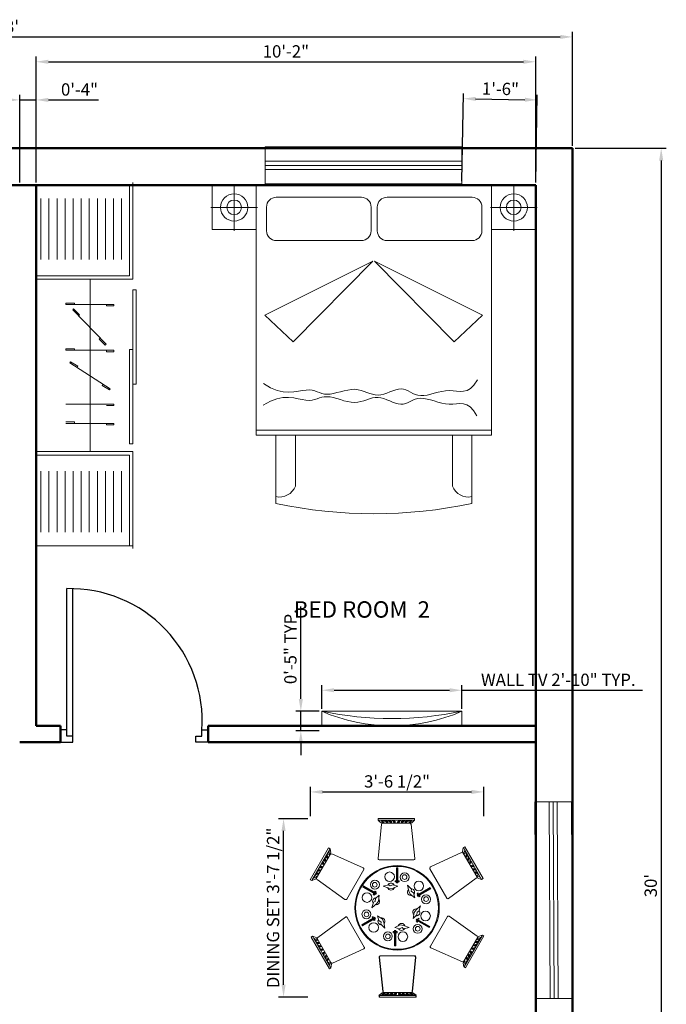
# Model space of a CAD drawing. Units: inches. Extents: x 108 to 1546, y -229 to 513.
# Tile 3 of 11: x 274 to 432, y 147 to 388. Entities that reach past the tile are written whole.
import ezdxf

# ---------------------------------------------------------------- set-up
doc = ezdxf.new("R2010")
doc.units = ezdxf.units.IN
for name, color, linetype, lineweight in [('A-ANNO-DIMS', 2, 'Continuous', 18), ('A-AREA-IDEN', 4, 'Continuous', 18), ('A-FURN', 8, 'Continuous', 13), ('door', 1, 'Continuous', 25), ('tv', 2, 'Continuous', 13), ('wall', 7, 'Continuous', 50), ('WINDOW', 212, 'Continuous', 18)]:
    doc.layers.add(name, color=color, linetype=linetype, lineweight=lineweight)
doc.styles.get("Standard").update_dxf_attribs({"font": 'arial.ttf'})
doc.dimstyles.new('ISO-25', dxfattribs={"dimtxt": 3, "dimasz": 3, "dimexe": 1.25, "dimexo": 0.625, "dimtad": 1, "dimdec": 1, "dimlunit": 3, "dimtxsty": 'Standard', "dimcen": 2.5, "dimadec": 0, "dimazin": 0, "dimtfac": 1, "dimtdec": 1, "dimtmove": 0, "dimatfit": 3, "dimfxl": 1, "dimarcsym": 0})

# ---------------------------------------------------------------- blocks, each defined once
blk = doc.blocks.new('A$C4F543DC7')
for p, q in [((0.013, 3.35, -0.169), (3.313, 3.35, -0.169)), ((0.463, 3.35, -0.169), (0.013, 3.35, -0.169)), ((0.013, 2.896, -0.169), (0.013, 3.35, -0.169)), ((0.013, 3.35, -0.169), (0.013, 2.896, -0.169)), ((0.238, 3.123, -0.439), (0.238, 3.361, -0.439)), ((0.463, 3.35, -0.169), (0.463, 0.8, -0.169)), ((2.863, 3.35, -0.169), (0.463, 3.35, -0.169)), ((0.463, 2.896, -0.169), (0.463, 3.35, -0.169)), ((2.863, 0.8, -0.169), (2.863, 3.35, -0.169)), ((2.863, 3.35, -0.169), (3.313, 3.35, -0.169)), ((2.863, 2.896, -0.169), (2.863, 3.35, -0.169)), ((3.089, 3.123, -0.439), (3.089, 3.361, -0.439)), ((3.313, 3.35, -0.169), (3.313, 2.896, -0.169)), ((3.313, 3.35, -0.169), (3.313, 2.896, -0.169)), ((1.535, 3.226, -0.169), (0.668, 3.226, -0.169)), ((2.664, 3.226, -0.169), (1.797, 3.226, -0.169)), ((0.238, 3.123, -0.439), (0, 3.123, -0.439)), ((0.238, 3.123, -0.439), (0.476, 3.123, -0.439)), ((0.238, 3.123, -0.439), (0.238, 2.885, -0.439)), ((0.568, 3.126, -0.169), (0.568, 2.884, -0.169)), ((1.635, 2.884, -0.169), (1.635, 3.126, -0.169)), ((1.697, 3.126, -0.169), (1.697, 2.884, -0.169)), ((2.764, 2.884, -0.169), (2.764, 3.126, -0.169)), ((3.089, 3.123, -0.439), (2.851, 3.123, -0.439)), ((3.089, 3.123, -0.439), (3.089, 2.885, -0.439)), ((3.089, 3.123, -0.439), (3.327, 3.123, -0.439)), ((0.463, 2.896, -0.169), (0.013, 2.896, -0.169)), ((0.013, 2.896, -0.169), (0.463, 2.896, -0.169)), ((0.463, 0.8, -0.169), (0.463, 2.896, -0.169)), ((2.863, 2.896, -0.169), (2.863, 0.8, -0.169)), ((3.313, 2.896, -0.169), (2.863, 2.896, -0.169)), ((3.313, 2.896, -0.169), (2.863, 2.896, -0.169)), ((0.668, 2.784, -0.169), (1.535, 2.784, -0.169)), ((1.797, 2.784, -0.169), (2.664, 2.784, -0.169)), ((1.653, 2.573, -0.169), (0.55, 2.025, -0.169)), ((0.841, 1.752, -0.169), (1.653, 2.573, -0.169)), ((2.481, 1.752, -0.169), (1.669, 2.573, -0.169)), ((1.669, 2.573, -0.169), (2.772, 2.025, -0.169)), ((0.55, 2.025, -0.169), (0.841, 1.752, -0.169)), ((2.772, 2.025, -0.169), (2.481, 1.752, -0.169)), ((0.537, 1.327, -0.169), (0.609, 1.284, -0.169)), ((2.648, 1.277, -0.169), (2.683, 1.312, -0.169)), ((2.683, 1.312, -0.169), (2.718, 1.364, -0.169)), ((0.609, 1.284, -0.169), (0.676, 1.257, -0.169)), ((0.676, 1.257, -0.169), (0.737, 1.243, -0.169)), ((0.737, 1.243, -0.169), (0.794, 1.239, -0.169)), ((0.794, 1.239, -0.169), (0.846, 1.242, -0.169)), ((0.846, 1.242, -0.169), (0.893, 1.249, -0.169)), ((0.893, 1.249, -0.169), (0.935, 1.256, -0.169)), ((0.935, 1.256, -0.169), (0.972, 1.261, -0.169)), ((0.972, 1.261, -0.169), (1.004, 1.262, -0.169)), ((1.004, 1.262, -0.169), (1.033, 1.258, -0.169)), ((1.033, 1.258, -0.169), (1.06, 1.251, -0.169)), ((1.06, 1.251, -0.169), (1.084, 1.242, -0.169)), ((1.084, 1.242, -0.169), (1.108, 1.234, -0.169)), ((1.108, 1.234, -0.169), (1.132, 1.226, -0.169)), ((1.132, 1.226, -0.169), (1.158, 1.22, -0.169)), ((1.158, 1.22, -0.169), (1.185, 1.218, -0.169)), ((1.185, 1.218, -0.169), (1.216, 1.22, -0.169)), ((1.216, 1.22, -0.169), (1.25, 1.226, -0.169)), ((1.25, 1.226, -0.169), (1.285, 1.235, -0.169)), ((1.285, 1.235, -0.169), (1.322, 1.244, -0.169)), ((1.322, 1.244, -0.169), (1.359, 1.253, -0.169)), ((1.359, 1.253, -0.169), (1.396, 1.261, -0.169)), ((1.396, 1.261, -0.169), (1.433, 1.266, -0.169)), ((1.433, 1.266, -0.169), (1.468, 1.268, -0.169)), ((1.468, 1.268, -0.169), (1.501, 1.264, -0.169)), ((1.501, 1.264, -0.169), (1.532, 1.257, -0.169)), ((1.532, 1.257, -0.169), (1.562, 1.247, -0.169)), ((1.562, 1.247, -0.169), (1.591, 1.237, -0.169)), ((1.591, 1.237, -0.169), (1.62, 1.226, -0.169)), ((1.62, 1.226, -0.169), (1.648, 1.217, -0.169)), ((1.648, 1.217, -0.169), (1.676, 1.211, -0.169)), ((1.676, 1.211, -0.169), (1.705, 1.209, -0.169)), ((1.705, 1.209, -0.169), (1.735, 1.212, -0.169)), ((1.735, 1.212, -0.169), (1.765, 1.22, -0.169)), ((1.765, 1.22, -0.169), (1.795, 1.23, -0.169)), ((1.795, 1.23, -0.169), (1.826, 1.242, -0.169)), ((1.826, 1.242, -0.169), (1.856, 1.253, -0.169)), ((1.856, 1.253, -0.169), (1.885, 1.263, -0.169)), ((1.885, 1.263, -0.169), (1.913, 1.27, -0.169)), ((1.913, 1.27, -0.169), (1.94, 1.272, -0.169)), ((1.94, 1.272, -0.169), (1.965, 1.269, -0.169)), ((1.965, 1.269, -0.169), (1.989, 1.262, -0.169)), ((1.989, 1.262, -0.169), (2.012, 1.251, -0.169)), ((2.012, 1.251, -0.169), (2.036, 1.239, -0.169)), ((2.036, 1.239, -0.169), (2.06, 1.227, -0.169)), ((2.06, 1.227, -0.169), (2.085, 1.216, -0.169)), ((2.085, 1.216, -0.169), (2.112, 1.208, -0.169)), ((2.112, 1.208, -0.169), (2.141, 1.204, -0.169)), ((2.141, 1.204, -0.169), (2.172, 1.205, -0.169)), ((2.172, 1.205, -0.169), (2.206, 1.21, -0.169)), ((2.206, 1.21, -0.169), (2.242, 1.218, -0.169)), ((2.242, 1.218, -0.169), (2.279, 1.228, -0.169)), ((2.279, 1.228, -0.169), (2.317, 1.238, -0.169)), ((2.317, 1.238, -0.169), (2.356, 1.246, -0.169)), ((2.356, 1.246, -0.169), (2.394, 1.253, -0.169)), ((2.394, 1.253, -0.169), (2.433, 1.255, -0.169)), ((2.433, 1.255, -0.169), (2.47, 1.253, -0.169)), ((2.47, 1.253, -0.169), (2.506, 1.249, -0.169)), ((2.506, 1.249, -0.169), (2.542, 1.246, -0.169)), ((2.542, 1.246, -0.169), (2.578, 1.248, -0.169)), ((2.578, 1.248, -0.169), (2.613, 1.257, -0.169)), ((2.613, 1.257, -0.169), (2.648, 1.277, -0.169)), ((0.533, 1.105, -0.169), (0.607, 1.146, -0.169)), ((0.607, 1.146, -0.169), (0.674, 1.171, -0.169)), ((0.674, 1.171, -0.169), (0.736, 1.183, -0.169)), ((0.736, 1.183, -0.169), (0.793, 1.185, -0.169)), ((0.793, 1.185, -0.169), (0.845, 1.18, -0.169)), ((0.845, 1.18, -0.169), (0.891, 1.172, -0.169)), ((0.891, 1.172, -0.169), (0.933, 1.163, -0.169)), ((0.933, 1.163, -0.169), (0.97, 1.156, -0.169)), ((0.97, 1.156, -0.169), (1.003, 1.155, -0.169)), ((1.003, 1.155, -0.169), (1.032, 1.158, -0.169)), ((1.032, 1.158, -0.169), (1.058, 1.164, -0.169)), ((1.058, 1.164, -0.169), (1.083, 1.172, -0.169)), ((1.083, 1.172, -0.169), (1.107, 1.18, -0.169)), ((1.107, 1.18, -0.169), (1.132, 1.187, -0.169)), ((1.132, 1.187, -0.169), (1.157, 1.192, -0.169)), ((1.157, 1.192, -0.169), (1.185, 1.193, -0.169)), ((1.185, 1.193, -0.169), (1.216, 1.19, -0.169)), ((1.216, 1.19, -0.169), (1.249, 1.183, -0.169)), ((1.249, 1.183, -0.169), (1.284, 1.173, -0.169)), ((1.284, 1.173, -0.169), (1.321, 1.163, -0.169)), ((1.321, 1.163, -0.169), (1.358, 1.152, -0.169)), ((1.358, 1.152, -0.169), (1.394, 1.143, -0.169)), ((1.394, 1.143, -0.169), (1.431, 1.137, -0.169)), ((1.431, 1.137, -0.169), (1.466, 1.135, -0.169)), ((1.466, 1.135, -0.169), (1.499, 1.137, -0.169)), ((1.499, 1.137, -0.169), (1.531, 1.143, -0.169)), ((1.531, 1.143, -0.169), (1.561, 1.152, -0.169)), ((1.561, 1.152, -0.169), (1.59, 1.162, -0.169)), ((1.59, 1.162, -0.169), (1.619, 1.172, -0.169)), ((1.619, 1.172, -0.169), (1.648, 1.18, -0.169)), ((1.648, 1.18, -0.169), (1.676, 1.185, -0.169)), ((1.676, 1.185, -0.169), (1.705, 1.186, -0.169)), ((1.705, 1.186, -0.169), (1.734, 1.182, -0.169)), ((1.734, 1.182, -0.169), (1.764, 1.173, -0.169)), ((1.764, 1.173, -0.169), (1.794, 1.162, -0.169)), ((1.794, 1.162, -0.169), (1.824, 1.149, -0.169)), ((1.824, 1.149, -0.169), (1.854, 1.137, -0.169)), ((1.854, 1.137, -0.169), (1.883, 1.126, -0.169)), ((1.883, 1.126, -0.169), (1.911, 1.119, -0.169)), ((1.911, 1.119, -0.169), (1.937, 1.115, -0.169)), ((1.937, 1.115, -0.169), (1.963, 1.118, -0.169)), ((1.963, 1.118, -0.169), (1.987, 1.124, -0.169)), ((1.987, 1.124, -0.169), (2.011, 1.134, -0.169)), ((2.011, 1.134, -0.169), (2.034, 1.145, -0.169)), ((2.034, 1.145, -0.169), (2.059, 1.157, -0.169)), ((2.059, 1.157, -0.169), (2.084, 1.167, -0.169)), ((2.084, 1.167, -0.169), (2.111, 1.174, -0.169)), ((2.111, 1.174, -0.169), (2.14, 1.177, -0.169)), ((2.14, 1.177, -0.169), (2.172, 1.175, -0.169)), ((2.172, 1.175, -0.169), (2.206, 1.169, -0.169)), ((2.206, 1.169, -0.169), (2.241, 1.16, -0.169)), ((2.241, 1.16, -0.169), (2.278, 1.149, -0.169)), ((2.278, 1.149, -0.169), (2.316, 1.138, -0.169)), ((2.316, 1.138, -0.169), (2.354, 1.128, -0.169)), ((2.354, 1.128, -0.169), (2.392, 1.121, -0.169)), ((2.392, 1.121, -0.169), (2.43, 1.117, -0.169)), ((2.43, 1.117, -0.169), (2.468, 1.118, -0.169)), ((2.468, 1.118, -0.169), (2.504, 1.121, -0.169)), ((2.504, 1.121, -0.169), (2.54, 1.123, -0.169)), ((2.54, 1.123, -0.169), (2.576, 1.12, -0.169)), ((2.576, 1.12, -0.169), (2.611, 1.109, -0.169)), ((2.611, 1.109, -0.169), (2.645, 1.088, -0.169)), ((2.645, 1.088, -0.169), (2.679, 1.052, -0.169)), ((2.679, 1.052, -0.169), (2.712, 0.999, -0.169)), ((0.463, 0.85, -0.169), (2.863, 0.85, -0.169)), ((0.463, 0.8, -0.169), (2.863, 0.8, -0.169)), ((0.663, 0.8, -0.169), (0.463, 0.8, -0.169)), ((0.663, 0.8, -0.169), (2.663, 0.8, -0.169)), ((0.663, 0.104, -0.169), (0.663, 0.8, -0.169)), ((0.663, 0.104, -0.169), (0.663, 0.8, -0.169)), ((0.863, 0.281, -0.169), (0.863, 0.8, -0.169)), ((2.463, 0.8, -0.169), (2.463, 0.281, -0.169)), ((2.863, 0.8, -0.169), (2.663, 0.8, -0.169)), ((2.663, 0.8, -0.169), (2.663, 0.104, -0.169)), ((2.663, 0.8, -0.169), (2.663, 0.104, -0.169))]:
    blk.add_line(p, q)
for centre, radius in [((0.238, 3.123, -0.439), 0.139), ((3.089, 3.123, -0.439), 0.139), ((0.238, 3.123, -0.439), 0.075), ((3.089, 3.123, -0.439), 0.075)]:
    blk.add_circle(centre, radius)
for centre, radius, start, end in [((0.668, 3.126, -0.169), 0.1, 90, 180), ((1.535, 3.126, -0.169), 0.1, 0, 90), ((1.797, 3.126, -0.169), 0.1, 90, 180), ((2.664, 3.126, -0.169), 0.1, 0, 90), ((0.668, 2.884, -0.169), 0.1, 180, 270), ((1.535, 2.884, -0.169), 0.1, 270, 0), ((1.797, 2.884, -0.169), 0.1, 180, 270), ((2.664, 2.884, -0.169), 0.1, 270, 0), ((0.699, 0.347, -0.169), 0.177, 258.2616, 338.032), ((2.627, 0.347, -0.169), 0.177, 201.968, 281.7384), ((1.663, 4.86, -0.169), 4.86, 258.1252, 281.8748), ((1.663, 4.86, -0.169), 4.86, 258.1252, 281.8748)]:
    blk.add_arc(centre, radius, start, end)
blk = doc.blocks.new('A$C34930FF8')
for p, q in [((600, 1669.3), (600, 2269.3)), ((580, 1690.9), (580, 2252.4)), ((30, 1790.9), (30, 2169.3)), ((80, 1790.9), (80, 2169.3)), ((130, 1790.9), (130, 2169.3)), ((180, 1790.9), (180, 2169.3)), ((230, 1790.9), (230, 2169.3)), ((280, 1790.9), (280, 2169.3)), ((330, 1790.9), (330, 2169.3)), ((380, 1790.9), (380, 2169.3)), ((430, 1790.9), (430, 2169.3)), ((480, 1790.9), (480, 2169.3)), ((530, 1790.9), (530, 2169.3)), ((580, 1690.9), (0, 1690.9)), ((600, 1669.3), (0, 1669.3)), ((335.4, 1666.1), (335.4, 603.1)), ((600, 1603.3), (620, 1603.3)), ((600, 1018.7), (600, 1603.3)), ((620, 1603.3), (620, 1018.7)), ((237.7, 1521.5), (185.4, 1521.5)), ((482.5, 1513), (185.4, 1513)), ((434.8, 1266.1), (227.4, 1478.9)), ((269.7, 1447.7), (233.2, 1485.2)), ((436.7, 1504.4), (482.5, 1504.4)), ((428.7, 1260.1), (392.1, 1297.6)), ((237.7, 1237.7), (185.4, 1237.7)), ((482.5, 1228.2), (185.4, 1228.2)), ((600, 1233.4), (580, 1233.4)), ((580, 1233.4), (580, 648.7)), ((600, 648.7), (600, 1233.4)), ((436.7, 1219.7), (482.5, 1219.7)), ((459.3, 989.3), (209.5, 1150.1)), ((258.1, 1129), (214.1, 1157.3)), ((454.7, 982.1), (410.6, 1010.5)), ((620, 1018.7), (600, 1018.7)), ((482.5, 894.9), (185.4, 894.9)), ((436.7, 886.3), (482.5, 886.3)), ((237.7, 783.9), (185.4, 783.9)), ((482.5, 775.3), (185.4, 775.3)), ((436.7, 766.8), (482.5, 766.8)), ((580, 648.7), (600, 648.7)), ((600, 600), (0, 600)), ((580, 578.3), (0, 578.3)), ((580, 578.3), (580, 16.8)), ((600, 600), (600, 0)), ((30, 478.3), (30, 100)), ((80, 478.3), (80, 100)), ((130, 478.3), (130, 100)), ((180, 478.3), (180, 100)), ((230, 478.3), (230, 100)), ((280, 478.3), (280, 100)), ((330, 478.3), (330, 100)), ((380, 478.3), (380, 100)), ((430, 478.3), (430, 100)), ((480, 478.3), (480, 100)), ((530, 478.3), (530, 100))]:
    blk.add_line(p, q)
at = {"ltscale": 0.05}
for p, q in [((0, 2252.4), (0, 16.8)), ((600, 2252.4), (0, 2252.4)), ((185.4, 1513), (185.4, 1521.5)), ((227.1, 1479.2), (233.2, 1485.2)), ((237.7, 1513), (237.7, 1521.5)), ((436.7, 1513), (436.7, 1504.4)), ((482.5, 1513), (482.5, 1504.4)), ((263.6, 1441.7), (269.7, 1447.7)), ((398.2, 1303.6), (392.1, 1297.6)), ((185.4, 1229.1), (185.4, 1237.7)), ((237.7, 1229.1), (237.7, 1237.7)), ((434.8, 1266.1), (428.7, 1260.1)), ((436.7, 1228.2), (436.7, 1219.7)), ((482.5, 1228.2), (482.5, 1219.7)), ((209.5, 1150.1), (214.1, 1157.3)), ((253.5, 1121.8), (258.1, 1129)), ((415.3, 1017.6), (410.6, 1010.5)), ((459.3, 989.3), (454.7, 982.1)), ((482.5, 894.9), (482.5, 886.3)), ((237.7, 775.3), (237.7, 783.9)), ((436.7, 775.3), (436.7, 766.8)), ((482.5, 775.3), (482.5, 766.8)), ((600, 16.8), (0, 16.8))]:
    blk.add_line(p, q, dxfattribs=at)
blk = doc.blocks.new('A$C45501D90')
for p, q in [((-242, 1134), (224, 1134)), ((-242, 1113), (-242, 1134)), ((224, 1134), (224, 1113)), ((224, 1113), (-242, 1113)), ((-242, 1111), (-202, 1079)), ((-197, 1062), (-239, 628)), ((-204, 1106), (-166, 1108)), ((-169, 1081), (-204, 1106)), ((-202, 1079), (-169, 1081)), ((162, 1076), (-181, 1076)), ((-166, 1108), (-167, 1086)), ((-156, 1110), (-132, 1086)), ((-119, 1086), (-143, 1108)), ((-143, 1108), (-134, 1108)), ((-134, 1108), (-122, 1098)), ((-132, 1086), (-119, 1086)), ((-122, 1098), (-119, 1102)), ((-119, 1102), (-118, 1087)), ((-108, 1110), (-84, 1086)), ((-71, 1086), (-95, 1108)), ((-95, 1108), (-86, 1108)), ((-86, 1108), (-75, 1098)), ((-84, 1086), (-71, 1086)), ((-75, 1098), (-71, 1102)), ((-71, 1102), (-70, 1087)), ((-60, 1110), (-36, 1086)), ((-23, 1086), (-47, 1108)), ((-47, 1108), (-38, 1108)), ((-38, 1108), (-27, 1098)), ((-36, 1086), (-23, 1086)), ((-27, 1098), (-23, 1102)), ((-23, 1102), (-22, 1087)), ((8, 1102), (7, 1087)), ((8, 1086), (32, 1108)), ((12, 1098), (8, 1102)), ((21, 1086), (8, 1086)), ((23, 1108), (12, 1098)), ((45, 1110), (21, 1086)), ((32, 1108), (23, 1108)), ((56, 1102), (55, 1087)), ((56, 1086), (80, 1108)), ((60, 1098), (56, 1102)), ((69, 1086), (56, 1086)), ((71, 1108), (60, 1098)), ((93, 1110), (69, 1086)), ((80, 1108), (71, 1108)), ((104, 1102), (103, 1087)), ((104, 1086), (128, 1108)), ((107, 1098), (104, 1102)), ((117, 1086), (104, 1086)), ((119, 1108), (107, 1098)), ((141, 1110), (117, 1086)), ((128, 1108), (119, 1108)), ((189, 1106), (151, 1108)), ((151, 1108), (152, 1086)), ((154, 1081), (189, 1106)), ((187, 1079), (154, 1081)), ((225, 628), (178, 1062)), ((224, 1113), (187, 1079)), ((-1103, 357), (-870, 761)), ((-870, 761), (-852, 750)), ((-849, 752), (-841, 702)), ((841, 765), (834, 715)), ((843, 766), (861, 776)), ((1076, 362), (843, 766)), ((861, 776), (1094, 373)), ((-852, 750), (-1085, 347)), ((-851, 678), (-1023, 381)), ((-914, 635), (-906, 603)), ((-898, 642), (-902, 641)), ((-902, 641), (-890, 633)), ((-895, 665), (-900, 657)), ((-900, 657), (-898, 642)), ((-888, 633), (-895, 665)), ((-890, 677), (-882, 644)), ((-882, 644), (-888, 633)), ((-864, 717), (-884, 684)), ((-884, 684), (-864, 675)), ((-859, 674), (-864, 717)), ((-841, 702), (-859, 674)), ((-431, 509), (-831, 685)), ((821, 702), (424, 521)), ((834, 715), (852, 687)), ((1013, 398), (841, 695)), ((852, 687), (856, 730)), ((856, 730), (877, 697)), ((877, 697), (857, 688)), ((883, 690), (874, 657)), ((874, 657), (881, 646)), ((881, 646), (888, 678)), ((894, 654), (883, 646)), ((888, 678), (893, 670)), ((893, 670), (890, 655)), ((890, 655), (894, 654)), ((907, 648), (898, 616)), ((904, 605), (912, 637)), ((912, 637), (917, 628)), ((917, 628), (914, 614)), ((-991, 503), (-958, 511)), ((-952, 522), (-983, 513)), ((-983, 513), (-978, 521)), ((-978, 521), (-965, 526)), ((-965, 526), (-966, 530)), ((-966, 530), (-953, 525)), ((-958, 511), (-952, 522)), ((-945, 559), (-950, 558)), ((-950, 558), (-938, 550)), ((-943, 582), (-948, 574)), ((-948, 574), (-945, 559)), ((-936, 550), (-943, 582)), ((-938, 594), (-930, 561)), ((-930, 561), (-936, 550)), ((-921, 601), (-926, 600)), ((-926, 600), (-914, 591)), ((-919, 624), (-924, 615)), ((-924, 615), (-921, 601)), ((-912, 592), (-919, 624)), ((-906, 603), (-912, 592)), ((-223, 610), (209, 610)), ((-6, 509, 91), (0, 509, 91)), ((-6, 318, 91), (-6, 509, 91)), ((0, 509, 91), (0, 318, 91)), ((6, 318, 91), (6, 509, 91)), ((6, 509, 91), (12, 509, 91)), ((12, 509, 91), (12, 318, 91)), ((898, 616), (904, 605)), ((918, 613), (907, 604)), ((914, 614), (918, 613)), ((931, 607), (922, 574)), ((922, 574), (928, 563)), ((928, 563), (936, 595)), ((942, 571), (931, 563)), ((936, 595), (941, 587)), ((941, 587), (938, 572)), ((938, 572), (942, 571)), ((951, 524), (944, 535)), ((944, 535), (976, 526)), ((958, 543), (945, 538)), ((983, 516), (951, 524)), ((957, 539), (958, 543)), ((971, 534), (957, 539)), ((982, 502), (969, 496)), ((976, 526), (971, 534)), ((981, 498), (982, 502)), ((-1060, 377), (-1042, 411)), ((-1020, 394), (-1060, 377)), ((-1042, 411), (-1024, 398)), ((-1039, 420), (-1006, 428)), ((-1036, 364), (-1020, 394)), ((-1000, 440), (-1031, 430)), ((-1031, 430), (-1026, 438)), ((-1026, 438), (-1012, 443)), ((-1015, 461), (-982, 470)), ((-1012, 443), (-1014, 448)), ((-1014, 448), (-1000, 442)), ((-976, 481), (-1007, 471)), ((-1007, 471), (-1002, 480)), ((-1006, 428), (-1000, 440)), ((-1002, 480), (-989, 485)), ((-989, 485), (-990, 489)), ((-990, 489), (-976, 483)), ((-982, 470), (-976, 481)), ((-640, 112), (-424, 486)), ((417, 498), (633, 124)), ((656, 119), (1008, 377)), ((968, 494), (1000, 484)), ((975, 483), (968, 494)), ((1007, 474), (975, 483)), ((995, 493), (981, 498)), ((999, 441), (992, 453)), ((992, 453), (1024, 443)), ((1006, 461), (993, 455)), ((1000, 484), (995, 493)), ((1031, 433), (999, 441)), ((1005, 456), (1006, 461)), ((1019, 451), (1005, 456)), ((1028, 377), (1013, 407)), ((1013, 407), (1053, 390)), ((1035, 424), (1016, 411)), ((1024, 443), (1019, 451)), ((1076, 359), (1028, 377)), ((1053, 390), (1035, 424)), ((-1085, 347), (-1103, 357)), ((-1083, 346), (-1036, 364)), ((-1018, 360), (-663, 107)), ((-436, 265, 91), (-433, 271, 91)), ((-271, 170, 91), (-436, 265, 91)), ((-433, 271, 91), (-268, 175, 91)), ((-431, 275, 91), (-428, 280, 91)), ((-265, 180, 91), (-431, 275, 91)), ((-428, 280, 91), (-262, 185, 91)), ((-175, 276, 91), (-105, 293, 91)), ((-103, 252, 91), (-175, 276, 91)), ((-105, 293, 91), (-86, 278, 91)), ((-60, 246, 91), (-103, 252, 91)), ((-86, 278, 91), (-52, 294, 91)), ((9, 276, 91), (-60, 246, 91)), ((-52, 294, 91), (9, 276, 91)), ((-22, 329, 91), (-22, 345, 91)), ((-22, 345, 91), (-6, 345, 91)), ((-6, 329, 91), (-22, 329, 91)), ((0, 318, 91), (-6, 318, 91)), ((0, 345, 91), (6, 345, 91)), ((6, 329, 91), (0, 329, 91)), ((12, 318, 91), (6, 318, 91)), ((12, 345, 91), (27, 345, 91)), ((27, 329, 91), (12, 329, 91)), ((27, 345, 91), (27, 329, 91)), ((134, 288, 91), (184, 236, 91)), ((150, 214, 91), (134, 288, 91)), ((255, 162, 91), (421, 257, 91)), ((424, 252, 91), (258, 157, 91)), ((421, 257, 91), (424, 252, 91)), ((1094, 373), (1076, 362)), ((-303, 169, 91), (-294, 183, 91)), ((-289, 161, 91), (-303, 169, 91)), ((-291, 188, 91), (-289, 193, 91)), ((-281, 176, 91), (-289, 161, 91)), ((-286, 198, 91), (-278, 212, 91)), ((-278, 212, 91), (-264, 204, 91)), ((-275, 185, 91), (-278, 181, 91)), ((-274, 118, 91), (-227, 162, 91)), ((-264, 204, 91), (-272, 191, 91)), ((-268, 175, 91), (-271, 170, 91)), ((-262, 185, 91), (-265, 180, 91)), ((-227, 162, 91), (-236, 87, 91)), ((166, 173, 91), (150, 214, 91)), ((227, 128, 91), (166, 173, 91)), ((184, 236, 91), (181, 211, 91)), ((181, 211, 91), (211, 190, 91)), ((211, 190, 91), (227, 128, 91)), ((258, 157, 91), (255, 162, 91)), ((257, 182, 91), (270, 190, 91)), ((265, 168, 91), (257, 182, 91)), ((261, 152, 91), (426, 248, 91)), ((264, 147, 91), (261, 152, 91)), ((429, 242, 91), (264, 147, 91)), ((271, 158, 91), (268, 162, 91)), ((270, 190, 91), (278, 175, 91)), ((281, 139, 91), (274, 153, 91)), ((281, 170, 91), (284, 165, 91)), ((295, 147, 91), (281, 139, 91)), ((287, 160, 91), (295, 147, 91)), ((426, 248, 91), (429, 242, 91)), ((-320, 2, 91), (-299, 72, 91)), ((-263, 53, 91), (-320, 2, 91)), ((-299, 72, 91), (-277, 81, 91)), ((-277, 81, 91), (-274, 118, 91)), ((-236, 87, 91), (-263, 53, 91)), ((243, -25, 91), (299, 26, 91)), ((299, 26, 91), (279, -44, 91)), ((-656, -119), (-1008, -377)), ((-417, -498), (-633, -124)), ((-450, -214, 91), (-284, -119, 91)), ((-281, -124, 91), (-447, -220, 91)), ((-315, -119, 91), (-302, -111, 91)), ((-307, -132, 91), (-315, -119, 91)), ((-302, -111, 91), (-294, -125, 91)), ((-284, -119, 91), (-281, -124, 91)), ((-247, -100, 91), (-187, -145, 91)), ((-232, -162, 91), (-247, -100, 91)), ((207, -134, 91), (216, -60, 91)), ((253, -90, 91), (207, -134, 91)), ((216, -60, 91), (243, -25, 91)), ((256, -53, 91), (253, -90, 91)), ((279, -44, 91), (256, -53, 91)), ((640, -112), (424, -486)), ((1018, -360), (663, -107)), ((-447, -220, 91), (-450, -214, 91)), ((-444, -224, 91), (-279, -129, 91)), ((-441, -229, 91), (-444, -224, 91)), ((-276, -134, 91), (-441, -229, 91)), ((-302, -142, 91), (-304, -137, 91)), ((-290, -162, 91), (-299, -147, 91)), ((-291, -130, 91), (-288, -134, 91)), ((-277, -154, 91), (-290, -162, 91)), ((-285, -140, 91), (-277, -154, 91)), ((-279, -129, 91), (-276, -134, 91)), ((-201, -183, 91), (-232, -162, 91)), ((-205, -208, 91), (-201, -183, 91)), ((-155, -260, 91), (-205, -208, 91)), ((-187, -145, 91), (-170, -186, 91)), ((-170, -186, 91), (-155, -260, 91)), ((-30, -248, 91), (39, -218, 91)), ((32, -266, 91), (-30, -248, 91)), ((65, -250, 91), (32, -266, 91)), ((39, -218, 91), (83, -224, 91)), ((84, -265, 91), (65, -250, 91)), ((83, -224, 91), (155, -248, 91)), ((155, -248, 91), (84, -265, 91)), ((242, -157, 91), (245, -152, 91)), ((407, -252, 91), (242, -157, 91)), ((244, -176, 91), (252, -163, 91)), ((257, -184, 91), (244, -176, 91)), ((245, -152, 91), (410, -247, 91)), ((248, -147, 91), (251, -142, 91)), ((413, -243, 91), (248, -147, 91)), ((251, -142, 91), (416, -237, 91)), ((255, -157, 91), (257, -153, 91)), ((265, -170, 91), (257, -184, 91)), ((260, -148, 91), (269, -133, 91)), ((271, -160, 91), (268, -165, 91)), ((269, -133, 91), (282, -141, 91)), ((282, -141, 91), (274, -155, 91)), ((410, -247, 91), (407, -252, 91)), ((416, -237, 91), (413, -243, 91)), ((-1094, -373), (-1076, -362)), ((-861, -776), (-1094, -373)), ((-1076, -359), (-1028, -377)), ((-1076, -362), (-843, -766)), ((-48, -317, 91), (-48, -301, 91)), ((-48, -301, 91), (-32, -301, 91)), ((-32, -317, 91), (-48, -317, 91)), ((-32, -481, 91), (-32, -290, 91)), ((-32, -290, 91), (-26, -290, 91)), ((-26, -290, 91), (-26, -481, 91)), ((-26, -301, 91), (-21, -301, 91)), ((-21, -317, 91), (-26, -317, 91)), ((-21, -481, 91), (-21, -290, 91)), ((-21, -290, 91), (-15, -290, 91)), ((-15, -290, 91), (-15, -481, 91)), ((-15, -301, 91), (2, -301, 91)), ((2, -317, 91), (-15, -317, 91)), ((2, -301, 91), (2, -317, 91)), ((852, -750), (1085, -347)), ((1103, -357), (870, -761)), ((1036, -364), (1020, -394)), ((1083, -346), (1036, -364)), ((1085, -347), (1103, -357)), ((-1053, -390), (-1035, -424)), ((-1013, -407), (-1053, -390)), ((-1035, -424), (-1016, -411)), ((-1031, -433), (-999, -441)), ((-1028, -377), (-1013, -407)), ((-1024, -443), (-1019, -451)), ((-992, -453), (-1024, -443)), ((-1019, -451), (-1005, -456)), ((-1013, -398), (-841, -695)), ((-1007, -474), (-975, -483)), ((-1006, -461), (-993, -455)), ((-1005, -456), (-1006, -461)), ((-968, -494), (-1000, -484)), ((-1000, -484), (-995, -493)), ((-999, -441), (-992, -453)), ((-995, -493), (-981, -498)), ((-982, -502), (-969, -496)), ((-981, -498), (-982, -502)), ((-975, -483), (-968, -494)), ((-26, -481, 91), (-32, -481, 91)), ((-15, -481, 91), (-21, -481, 91)), ((851, -678), (1023, -381)), ((982, -470), (976, -481)), ((976, -481), (1007, -471)), ((990, -489), (976, -483)), ((1015, -461), (982, -470)), ((1002, -480), (989, -485)), ((989, -485), (990, -489)), ((1006, -428), (1000, -440)), ((1000, -440), (1031, -430)), ((1014, -448), (1000, -442)), ((1007, -471), (1002, -480)), ((1039, -420), (1006, -428)), ((1026, -438), (1012, -443)), ((1012, -443), (1014, -448)), ((1020, -394), (1060, -377)), ((1042, -411), (1024, -398)), ((1031, -430), (1026, -438)), ((1060, -377), (1042, -411)), ((-983, -516), (-951, -524)), ((-944, -535), (-976, -526)), ((-976, -526), (-971, -534)), ((-971, -534), (-957, -539)), ((-958, -543), (-945, -538)), ((-957, -539), (-958, -543)), ((-951, -524), (-944, -535)), ((-942, -571), (-931, -563)), ((-938, -572), (-942, -571)), ((-941, -587), (-938, -572)), ((-936, -595), (-941, -587)), ((-928, -563), (-936, -595)), ((-931, -607), (-922, -574)), ((-922, -574), (-928, -563)), ((-918, -613), (-907, -604)), ((-914, -614), (-918, -613)), ((-917, -628), (-914, -614)), ((-904, -605), (-912, -637)), ((-907, -648), (-898, -616)), ((-898, -616), (-904, -605)), ((-821, -702), (-424, -521)), ((219, -612), (-213, -612)), ((223, -610), (-209, -610)), ((431, -509), (831, -685)), ((906, -603), (912, -592)), ((914, -635), (906, -603)), ((912, -592), (919, -624)), ((926, -600), (914, -591)), ((919, -624), (924, -615)), ((921, -601), (926, -600)), ((924, -615), (921, -601)), ((930, -561), (936, -550)), ((938, -594), (930, -561)), ((936, -550), (943, -582)), ((950, -558), (938, -550)), ((943, -582), (948, -574)), ((945, -559), (950, -558)), ((948, -574), (945, -559)), ((958, -511), (952, -522)), ((952, -522), (983, -513)), ((966, -530), (953, -525)), ((991, -503), (958, -511)), ((978, -521), (965, -526)), ((965, -526), (966, -530)), ((983, -513), (978, -521)), ((-912, -637), (-917, -628)), ((-894, -654), (-883, -646)), ((-890, -655), (-894, -654)), ((-893, -670), (-890, -655)), ((-888, -678), (-893, -670)), ((-881, -646), (-888, -678)), ((-883, -690), (-874, -657)), ((-874, -657), (-881, -646)), ((-877, -697), (-857, -688)), ((-856, -730), (-877, -697)), ((-852, -687), (-856, -730)), ((-834, -715), (-852, -687)), ((-841, -765), (-834, -715)), ((-229, -629), (-182, -1063)), ((-225, -628), (-178, -1062)), ((193, -1063), (235, -629)), ((197, -1062), (239, -628)), ((841, -702), (859, -674)), ((849, -752), (841, -702)), ((870, -761), (852, -750)), ((859, -674), (864, -717)), ((884, -684), (864, -675)), ((864, -717), (884, -684)), ((882, -644), (888, -633)), ((890, -677), (882, -644)), ((888, -633), (895, -665)), ((902, -641), (890, -633)), ((895, -665), (900, -657)), ((898, -642), (902, -641)), ((900, -657), (898, -642)), ((-843, -766), (-861, -776)), ((-231, -1113), (-191, -1081)), ((-228, -1114), (238, -1114)), ((-228, -1135), (-228, -1114)), ((-227, -1111), (-187, -1079)), ((-224, -1113), (242, -1113)), ((-224, -1134), (-224, -1113)), ((-158, -1082), (-193, -1108)), ((-193, -1108), (-155, -1109)), ((-191, -1081), (-158, -1082)), ((-154, -1081), (-189, -1106)), ((-189, -1106), (-151, -1108)), ((-187, -1079), (-154, -1081)), ((-166, -1078), (177, -1078)), ((-162, -1076), (181, -1076)), ((-155, -1109), (-156, -1087)), ((-151, -1108), (-152, -1086)), ((-145, -1111), (-121, -1087)), ((-141, -1110), (-117, -1086)), ((-108, -1087), (-132, -1109)), ((-132, -1109), (-123, -1109)), ((-104, -1086), (-128, -1108)), ((-128, -1108), (-119, -1108)), ((-123, -1109), (-112, -1100)), ((-121, -1087), (-108, -1087)), ((-119, -1108), (-107, -1098)), ((-117, -1086), (-104, -1086)), ((-112, -1100), (-108, -1103)), ((-108, -1103), (-107, -1089)), ((-107, -1098), (-104, -1102)), ((-104, -1102), (-103, -1087)), ((-97, -1111), (-73, -1087)), ((-93, -1110), (-69, -1086)), ((-60, -1087), (-84, -1109)), ((-84, -1109), (-75, -1109)), ((-56, -1086), (-80, -1108)), ((-80, -1108), (-71, -1108)), ((-75, -1109), (-64, -1100)), ((-73, -1087), (-60, -1087)), ((-71, -1108), (-60, -1098)), ((-69, -1086), (-56, -1086)), ((-64, -1100), (-60, -1103)), ((-60, -1103), (-59, -1089)), ((-60, -1098), (-56, -1102)), ((-56, -1102), (-55, -1087)), ((-49, -1111), (-25, -1087)), ((-45, -1110), (-21, -1086)), ((-13, -1087), (-37, -1109)), ((-37, -1109), (-27, -1109)), ((-8, -1086), (-32, -1108)), ((-32, -1108), (-23, -1108)), ((-27, -1109), (-16, -1100)), ((-25, -1087), (-13, -1087)), ((-23, -1108), (-12, -1098)), ((-21, -1086), (-8, -1086)), ((-16, -1100), (-13, -1103)), ((-13, -1103), (-11, -1089)), ((-12, -1098), (-8, -1102)), ((-8, -1102), (-7, -1087)), ((19, -1103), (18, -1089)), ((19, -1087), (43, -1109)), ((32, -1087), (19, -1087)), ((23, -1100), (19, -1103)), ((23, -1102), (22, -1087)), ((23, -1086), (47, -1108)), ((36, -1086), (23, -1086)), ((27, -1098), (23, -1102)), ((34, -1109), (23, -1100)), ((38, -1108), (27, -1098)), ((56, -1111), (32, -1087)), ((43, -1109), (34, -1109)), ((60, -1110), (36, -1086)), ((47, -1108), (38, -1108)), ((67, -1103), (66, -1089)), ((67, -1087), (91, -1109)), ((80, -1087), (67, -1087)), ((70, -1100), (67, -1103)), ((71, -1102), (70, -1087)), ((82, -1109), (70, -1100)), ((71, -1086), (95, -1108)), ((84, -1086), (71, -1086)), ((75, -1098), (71, -1102)), ((86, -1108), (75, -1098)), ((104, -1111), (80, -1087)), ((91, -1109), (82, -1109)), ((108, -1110), (84, -1086)), ((95, -1108), (86, -1108)), ((115, -1103), (114, -1089)), ((115, -1087), (139, -1109)), ((128, -1087), (115, -1087)), ((118, -1100), (115, -1103)), ((119, -1102), (118, -1087)), ((130, -1109), (118, -1100)), ((119, -1086), (143, -1108)), ((132, -1086), (119, -1086)), ((122, -1098), (119, -1102)), ((134, -1108), (122, -1098)), ((152, -1111), (128, -1087)), ((139, -1109), (130, -1109)), ((156, -1110), (132, -1086)), ((143, -1108), (134, -1108)), ((161, -1109), (163, -1087)), ((200, -1108), (161, -1109)), ((198, -1081), (165, -1082)), ((165, -1082), (200, -1108)), ((166, -1108), (167, -1086)), ((204, -1106), (166, -1108)), ((202, -1079), (169, -1081)), ((169, -1081), (204, -1106)), ((238, -1113), (198, -1081)), ((242, -1111), (202, -1079)), ((238, -1114), (238, -1135)), ((242, -1113), (242, -1134)), ((238, -1135), (-228, -1135)), ((242, -1134), (-224, -1134))]:
    blk.add_line(p, q)
for centre, radius in [((0, 0), 537), ((0, 0), 527), ((-95, 395, 91), 61.3), ((97, 390, 91), 56.9), ((96, 391, 91), 29.4), ((-282, 295, 91), 56.9), ((-284, 294, 91), 29.4), ((277, 278, 91), 61.3), ((-382, 131, 91), 61.3), ((369, 109, 91), 56.9), ((369, 111, 91), 29.4), ((-389, -81, 91), 56.9), ((-389, -83, 91), 29.4), ((362, -103, 91), 61.3), ((-298, -250, 91), 61.3), ((262, -267, 91), 56.9), ((263, -266, 91), 29.4), ((-117, -362, 91), 56.9), ((-116, -363, 91), 29.4), ((74, -367, 91), 61.3)]:
    blk.add_circle(centre, radius)
for centre, radius, start, end in [((-181, 1060), 16, 90, 174.5199), ((162, 1060), 16, 6.2572, 90), ((-837, 670), 16, 66.2572, 150), ((-223, 626), 16, 174.5199, 270), ((209, 626), 16, 270, 6.2572), ((827, 687), 16, 30, 114.5199), ((-438, 494), 16, 330, 66.2572), ((431, 506), 16, 114.5199, 210), ((-1009, 373), 16, 150, 234.5199), ((999, 390), 16, 306.2572, 30), ((-77, 270, 91), 44.6, 195.9338, 342.9389), ((-77, 270, 91), 44.6, 25.8558, 153.3359), ((-266, 84, 91), 44.6, 85.8558, 213.3359), ((178, 200, 91), 44.6, 135.9338, 282.9389), ((178, 200, 91), 44.6, 325.8558, 93.3359), ((-654, 120), 16, 234.5199, 330), ((-266, 84, 91), 44.6, 255.9338, 42.9389), ((647, 132), 16, 210, 306.2572), ((-647, -132), 16, 30, 126.2572), ((245, -56, 91), 44.6, 75.9338, 222.9389), ((245, -56, 91), 44.6, 265.8558, 33.3359), ((654, -120), 16, 54.5199, 150), ((-198, -172, 91), 44.6, 145.8558, 273.3359), ((-198, -172, 91), 44.6, 315.9338, 102.9389), ((57, -242, 91), 44.6, 15.9338, 162.9389), ((57, -242, 91), 44.6, 205.8558, 333.3359), ((1009, -373), 16, 330, 54.5199), ((-999, -390), 16, 126.2572, 210), ((-431, -506), 16, 294.5199, 30), ((438, -494), 16, 150, 246.2572), ((-213, -628), 16, 90, 186.2572), ((-209, -626), 16, 90, 186.2572), ((219, -628), 16, 354.5199, 90), ((223, -626), 16, 354.5199, 90), ((-827, -687), 16, 210, 294.5199), ((837, -670), 16, 246.2572, 330), ((-166, -1062), 16, 186.2572, 270), ((-162, -1060), 16, 186.2572, 270), ((177, -1062), 16, 270, 354.5199), ((181, -1060), 16, 270, 354.5199)]:
    blk.add_arc(centre, radius, start, end)
blk = doc.blocks.new('*D21')
at = {"layer": 'A-ANNO-DIMS', "color": 0, "lineweight": -2, "transparency": 16777216}
for p, q in [((132.92, 357.09), (132.92, 384.9)), ((408.92, 357.09), (408.92, 384.9)), ((135.92, 383.65), (405.92, 383.65))]:
    blk.add_line(p, q, dxfattribs=at)
at = {"layer": 'A-ANNO-DIMS', "color": 0, "transparency": 16777216}
for points in [[(135.92, 384.15), (135.92, 383.15), (132.92, 383.65)], [(405.92, 384.15), (405.92, 383.15), (408.92, 383.65)]]:
    blk.add_solid(points, dxfattribs=at)
at = {"layer": 'Defpoints', "color": 0, "transparency": 16777216}
for p in [(408.92, 383.65), (132.92, 356.47), (408.92, 356.47)]:
    blk.add_point(p, dxfattribs=at)
at = {"layer": 'A-ANNO-DIMS', "color": 0, "transparency": 16777216, "insert": (270.92, 385.81), "char_height": 3, "attachment_point": 5}
blk.add_mtext("23'", dxfattribs=at)
blk = doc.blocks.new('*D22')
at = {"layer": 'A-ANNO-DIMS', "color": 0, "lineweight": -2, "transparency": 16777216}
for p, q in [((409.55, 356.47), (431.8, 356.47)), ((430.55, 353.47), (430.55, -0.53)), ((409.55, -3.53), (431.8, -3.53))]:
    blk.add_line(p, q, dxfattribs=at)
at = {"layer": 'A-ANNO-DIMS', "color": 0, "transparency": 16777216}
for points in [[(430.05, 353.47), (431.05, 353.47), (430.55, 356.47)], [(430.05, -0.53), (431.05, -0.53), (430.55, -3.53)]]:
    blk.add_solid(points, dxfattribs=at)
at = {"layer": 'Defpoints', "color": 0, "transparency": 16777216}
for p in [(408.92, 356.47), (408.92, -3.53), (430.55, -3.53)]:
    blk.add_point(p, dxfattribs=at)
at = {"layer": 'A-ANNO-DIMS', "color": 0, "transparency": 16777216, "insert": (428.39, 176.47), "char_height": 3, "attachment_point": 5, "rotation": 90}
blk.add_mtext("30'", dxfattribs=at)
blk = doc.blocks.new('WINDOW-48X9')
for p, q in [((0, 9), (0, 0)), ((0, 9), (48, 9)), ((48, 9), (48, 0)), ((0, 5.5), (48, 5.5)), ((0, 4.5), (48, 4.5)), ((0, 3.5), (48, 3.5)), ((0, 0), (48, 0))]:
    blk.add_line(p, q)
blk = doc.blocks.new('DOOR-SWING-36')
for p, q in [((1.5, 1.5), (1.5, 37.5)), ((3, 1.5), (3, 37.5)), ((0, 3), (0, 0)), ((1.5, 3), (0, 3)), ((1.5, 1.5), (1.5, 3)), ((34.5, 1.5), (34.5, 3)), ((34.5, 3), (36, 3)), ((36, 3), (36, 0)), ((3, 1.5), (1.5, 1.5)), ((3, 0), (3, 1.5)), ((33, 0), (33, 1.5)), ((33, 1.5), (34.5, 1.5)), ((0, 0), (3, 0)), ((36, 0), (33, 0))]:
    blk.add_line(p, q)
blk.add_arc((2.25, 5.18), 32.32, 356.1244, 91.3295)
blk = doc.blocks.new('TV-WALL-MOUNT')
blk.add_lwpolyline([(0, 0), (34.19, 0), (34.19, 3.56), (0, 3.56)], close=True)
for centre, radius, start, end in [((17.1, 42.8), 42.8, 246.4582, 293.5418), ((17.1, 84.72), 82.93, 258.1036, 281.8964)]:
    blk.add_arc(centre, radius, start, end)
blk = doc.blocks.new('*D42')
at = {"layer": 'A-ANNO-DIMS', "color": 0, "lineweight": -2, "transparency": 16777216}
for p, q in [((347.7, 219.66), (347.7, 225.41)), ((350.7, 224.16), (378.89, 224.16)), ((381.89, 219.66), (381.89, 225.41)), ((381.89, 224.16), (425.98, 224.16))]:
    blk.add_line(p, q, dxfattribs=at)
at = {"layer": 'A-ANNO-DIMS', "color": 0, "transparency": 16777216}
for points in [[(350.7, 224.66), (350.7, 223.66), (347.7, 224.16)], [(378.89, 224.66), (378.89, 223.66), (381.89, 224.16)]]:
    blk.add_solid(points, dxfattribs=at)
at = {"layer": 'Defpoints', "color": 0, "transparency": 16777216}
for p in [(381.89, 224.16), (347.7, 219.03), (381.89, 219.03)]:
    blk.add_point(p, dxfattribs=at)
at = {"layer": 'A-ANNO-DIMS', "color": 0, "transparency": 16777216, "insert": (405.43, 226.32), "char_height": 3, "attachment_point": 5}
blk.add_mtext('WALL TV 2\'-10" TYP.', dxfattribs=at)
blk = doc.blocks.new('*D43')
at = {"layer": 'A-ANNO-DIMS', "color": 0, "lineweight": -2, "transparency": 16777216}
for p, q in [((342.57, 222.03), (342.57, 244.57)), ((347.07, 219.03), (341.32, 219.03)), ((342.57, 214.28), (342.57, 219.03)), ((347.07, 214.28), (341.32, 214.28)), ((342.57, 211.28), (342.57, 208.28))]:
    blk.add_line(p, q, dxfattribs=at)
at = {"layer": 'A-ANNO-DIMS', "color": 0, "transparency": 16777216}
for points in [[(342.07, 222.03), (343.07, 222.03), (342.57, 219.03)], [(342.07, 211.28), (343.07, 211.28), (342.57, 214.28)]]:
    blk.add_solid(points, dxfattribs=at)
at = {"layer": 'Defpoints', "color": 0, "transparency": 16777216}
for p in [(342.57, 219.03), (347.7, 219.03), (347.7, 214.28)]:
    blk.add_point(p, dxfattribs=at)
at = {"layer": 'A-ANNO-DIMS', "color": 0, "transparency": 16777216, "insert": (340.41, 234.8), "char_height": 3, "attachment_point": 5, "rotation": 90}
blk.add_mtext('0\'-5" TYP.', dxfattribs=at)
blk = doc.blocks.new('*D52')
at = {"layer": 'A-ANNO-DIMS', "color": 0, "lineweight": -2, "transparency": 16777216}
for p, q in [((344.26, 192.8), (337.1, 192.8)), ((338.35, 152.25), (338.35, 189.8)), ((344.26, 149.25), (337.1, 149.25))]:
    blk.add_line(p, q, dxfattribs=at)
at = {"layer": 'A-ANNO-DIMS', "color": 0, "transparency": 16777216}
for points in [[(337.85, 189.8), (338.85, 189.8), (338.35, 192.8)], [(337.85, 152.25), (338.85, 152.25), (338.35, 149.25)]]:
    blk.add_solid(points, dxfattribs=at)
at = {"layer": 'Defpoints', "color": 0, "transparency": 16777216}
for p in [(338.35, 192.8), (344.89, 192.8), (344.89, 149.25)]:
    blk.add_point(p, dxfattribs=at)
at = {"layer": 'A-ANNO-DIMS', "color": 0, "transparency": 16777216, "insert": (336.18, 171.03), "char_height": 3, "attachment_point": 5, "rotation": 90}
blk.add_mtext('DINING SET 3\'-7 1/2"', dxfattribs=at)
blk = doc.blocks.new('*D53')
at = {"layer": 'A-ANNO-DIMS', "color": 0, "lineweight": -2, "transparency": 16777216}
for p, q in [((344.89, 193.43), (344.89, 200.59)), ((387.23, 193.43), (387.23, 200.59)), ((347.89, 199.34), (384.23, 199.34))]:
    blk.add_line(p, q, dxfattribs=at)
at = {"layer": 'A-ANNO-DIMS', "color": 0, "transparency": 16777216}
for points in [[(347.89, 199.84), (347.89, 198.84), (344.89, 199.34)], [(384.23, 199.84), (384.23, 198.84), (387.23, 199.34)]]:
    blk.add_solid(points, dxfattribs=at)
at = {"layer": 'Defpoints', "color": 0, "transparency": 16777216}
for p in [(387.23, 199.34), (344.89, 192.8), (387.23, 192.8)]:
    blk.add_point(p, dxfattribs=at)
at = {"layer": 'A-ANNO-DIMS', "color": 0, "transparency": 16777216, "insert": (366.06, 201.51), "char_height": 3, "attachment_point": 5}
blk.add_mtext('3\'-6 1/2"', dxfattribs=at)
blk = doc.blocks.new('*D73')
at = {"layer": 'A-ANNO-DIMS', "color": 0, "lineweight": -2, "transparency": 16777216}
for p, q in [((277.92, 348.09), (277.92, 378.83)), ((280.92, 377.58), (396.92, 377.58)), ((399.92, 348.09), (399.92, 378.83))]:
    blk.add_line(p, q, dxfattribs=at)
at = {"layer": 'A-ANNO-DIMS', "color": 0, "transparency": 16777216}
for points in [[(280.92, 378.08), (280.92, 377.08), (277.92, 377.58)], [(396.92, 378.08), (396.92, 377.08), (399.92, 377.58)]]:
    blk.add_solid(points, dxfattribs=at)
at = {"layer": 'Defpoints', "color": 0, "transparency": 16777216}
for p in [(399.92, 377.58), (277.92, 347.47), (399.92, 347.47)]:
    blk.add_point(p, dxfattribs=at)
at = {"layer": 'A-ANNO-DIMS', "color": 0, "transparency": 16777216, "insert": (338.92, 379.73), "char_height": 3, "attachment_point": 5}
blk.add_mtext('10\'-2"', dxfattribs=at)
blk = doc.blocks.new('*D80')
at = {"layer": 'A-ANNO-DIMS', "color": 0, "lineweight": -2, "transparency": 16777216}
for p, q in [((270.92, 368.27), (267.92, 368.27)), ((273.92, 348.09), (273.92, 369.52)), ((273.92, 368.27), (277.92, 368.27)), ((277.92, 348.09), (277.92, 369.52)), ((280.92, 368.27), (293.15, 368.27))]:
    blk.add_line(p, q, dxfattribs=at)
at = {"layer": 'A-ANNO-DIMS', "color": 0, "transparency": 16777216}
for points in [[(270.92, 368.77), (270.92, 367.77), (273.92, 368.27)], [(280.92, 368.77), (280.92, 367.77), (277.92, 368.27)]]:
    blk.add_solid(points, dxfattribs=at)
at = {"layer": 'Defpoints', "color": 0, "transparency": 16777216}
for p in [(277.92, 368.27), (273.92, 347.47), (277.92, 347.47)]:
    blk.add_point(p, dxfattribs=at)
at = {"layer": 'A-ANNO-DIMS', "color": 0, "transparency": 16777216, "insert": (288.53, 370.43), "char_height": 3, "attachment_point": 5}
blk.add_mtext('0\'-4"', dxfattribs=at)
blk = doc.blocks.new('*D82')
at = {"layer": 'A-ANNO-DIMS', "color": 0, "lineweight": -2, "transparency": 16777216}
for p, q in [((381.9, 348.4), (382.27, 369.82)), ((385.25, 368.52), (397.28, 368.32)), ((399.93, 348.09), (400.3, 369.52))]:
    blk.add_line(p, q, dxfattribs=at)
at = {"layer": 'A-ANNO-DIMS', "color": 0, "transparency": 16777216}
for points in [[(385.26, 369.02), (385.24, 368.02), (382.25, 368.58)], [(397.29, 368.82), (397.27, 367.82), (400.28, 368.27)]]:
    blk.add_solid(points, dxfattribs=at)
at = {"layer": 'Defpoints', "color": 0, "transparency": 16777216}
for p in [(400.28, 368.27), (381.89, 347.78), (399.92, 347.47)]:
    blk.add_point(p, dxfattribs=at)
at = {"layer": 'A-ANNO-DIMS', "color": 0, "transparency": 16777216, "insert": (391.3, 370.58), "char_height": 3, "attachment_point": 5, "rotation": 359.0204}
blk.add_mtext('1\'-6"', dxfattribs=at)

msp = doc.modelspace()

# ---------------------------------------------------------------- linework, layer by layer
at = {"layer": 'wall'}
for p, q in [((408.92, 356.47), (132.92, 356.47)), ((408.92, -3.53), (408.92, 356.47)), ((399.92, 347.47), (141.92, 347.47)), ((277.92, 347.47), (277.92, 215.47)), ((399.92, 5.47), (399.92, 347.47)), ((283.92, 215.47), (277.92, 215.47)), ((283.92, 215.47), (283.92, 211.47)), ((399.92, 215.47), (319.92, 215.47)), ((319.92, 215.47), (319.92, 211.47)), ((283.92, 211.47), (273.92, 211.47)), ((399.92, 211.47), (319.92, 211.47))]:
    msp.add_line(p, q, dxfattribs=at)

# ---------------------------------------------------------------- block references
at = {"layer": 'A-FURN'}
for name, p, xscale, yscale, zscale in [('A$C34930FF8', (277.92, 258.79), 0.0393700787401575, 0.0393700787401575, 0.0393700787401575), ('A$C4F543DC7', (320.59, 267.26, 4.04), 23.94379789781286, 23.94379789781286, 23.94379789781286), ('A$C45501D90', (366.06, 171.04), 0.0191981613363788, 0.0191981613363788, 0.0191981613363788)]:
    msp.add_blockref(name, p, dxfattribs=dict(at, xscale=xscale, yscale=yscale, zscale=zscale))
at = {"layer": 'door'}
msp.add_blockref('DOOR-SWING-36', (283.92, 211.47), dxfattribs=at)
at = {"layer": 'tv'}
msp.add_blockref('TV-WALL-MOUNT', (347.7, 215.47), dxfattribs=at)
at = {"layer": 'WINDOW'}
for p, rotation in [((381.89, 356.78), 180), ((408.92, 148.93), 90.2799560098102)]:
    msp.add_blockref('WINDOW-48X9', p, dxfattribs=dict(at, rotation=rotation))

# ---------------------------------------------------------------- texts
at = {"layer": 'A-AREA-IDEN', "insert": (340.85, 245.88), "char_height": 4, "attachment_point": 1}
msp.add_mtext_dynamic_manual_height_columns('BED ROOM  2', width=57.4311, gutter_width=12.5, heights=[12.84], dxfattribs=at)

# ---------------------------------------------------------------- dimensions: what is measured, and where the dimension line sits
at = {"layer": 'A-ANNO-DIMS'}
for base, p1, p2, override, picture, middle in [((408.92, 383.65), (132.92, 356.47), (408.92, 356.47), {"dimclrd": 0, "dimclre": 0, "dimclrt": 0}, '*D21', (270.92, 385.81)), ((399.92, 377.58), (277.92, 347.47), (399.92, 347.47), {"dimdec": 1, "dimlfac": 1, "dimrnd": 0, "dimzin": 1, "dimdsep": 46, "dimlunit": 4, "dimfrac": 2}, '*D73', (338.92, 379.73)), ((277.92, 368.27), (273.92, 347.47), (277.92, 347.47), {"dimdec": 1, "dimlfac": 1, "dimrnd": 0, "dimzin": 1, "dimdsep": 46, "dimlunit": 4, "dimfrac": 2}, '*D80', (288.53, 370.43)), ((387.23, 199.34), (344.89, 192.8), (387.23, 192.8), {"dimdec": 1, "dimlfac": 1, "dimrnd": 0, "dimzin": 1, "dimdsep": 46, "dimlunit": 4, "dimfrac": 2}, '*D53', (366.06, 201.51))]:
    dim = msp.add_linear_dim(base=base, p1=p1, p2=p2, dimstyle='ISO-25', override=override, dxfattribs=at)
    dim.commit()
    dim.dimension.update_dxf_attribs({"geometry": picture, "text_midpoint": middle})
for base, p1, p2, angle, override, picture, middle in [((400.28, 368.27), (381.89, 347.78), (399.92, 347.47), 359.0204, {"dimdec": 1, "dimlfac": 1, "dimrnd": 0, "dimzin": 1, "dimdsep": 46, "dimlunit": 4, "dimfrac": 2}, '*D82', (391.3, 370.58)), ((430.55, -3.53), (408.92, 356.47), (408.92, -3.53), 90, {"dimclrd": 0, "dimclre": 0, "dimclrt": 0}, '*D22', (428.39, 176.47))]:
    dim = msp.add_linear_dim(base=base, p1=p1, p2=p2, angle=angle, dimstyle='ISO-25', override=override, dxfattribs=at)
    dim.commit()
    dim.dimension.update_dxf_attribs({"geometry": picture, "text_midpoint": middle})
for base, p1, p2, text, picture, middle in [((342.5684, 219.0325), (347.6973, 214.2824), (347.6973, 219.0325), '<> TYP.', '*D43', (340.4117, 234.8007)), ((338.3544, 192.8037), (344.8871, 149.2523), (344.8871, 192.8037), 'DINING SET <>', '*D52', (336.1772, 171.028))]:
    dim = msp.add_linear_dim(base=base, p1=p1, p2=p2, angle=90, text=text, dimstyle='ISO-25', override={"dimdec": 1, "dimlfac": 1, "dimrnd": 0, "dimzin": 1, "dimdsep": 46, "dimlunit": 4, "dimfrac": 2}, dxfattribs=at)
    dim.commit()
    dim.dimension.update_dxf_attribs({"geometry": picture, "text_midpoint": middle})
dim = msp.add_linear_dim(base=(381.89, 224.16), p1=(347.7, 219.03), p2=(381.89, 219.03), text='WALL TV <> TYP.', dimstyle='ISO-25', override={"dimdec": 1, "dimlfac": 1, "dimrnd": 0, "dimzin": 1, "dimdsep": 46, "dimlunit": 4, "dimfrac": 2}, dxfattribs=at)
dim.commit()
dim.dimension.update_dxf_attribs({"geometry": '*D42', "text_midpoint": (405.43, 226.32)})

doc.saveas('drawing.dxf')
